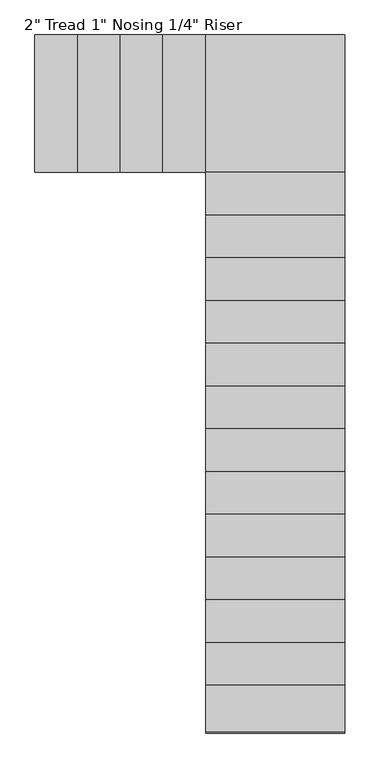
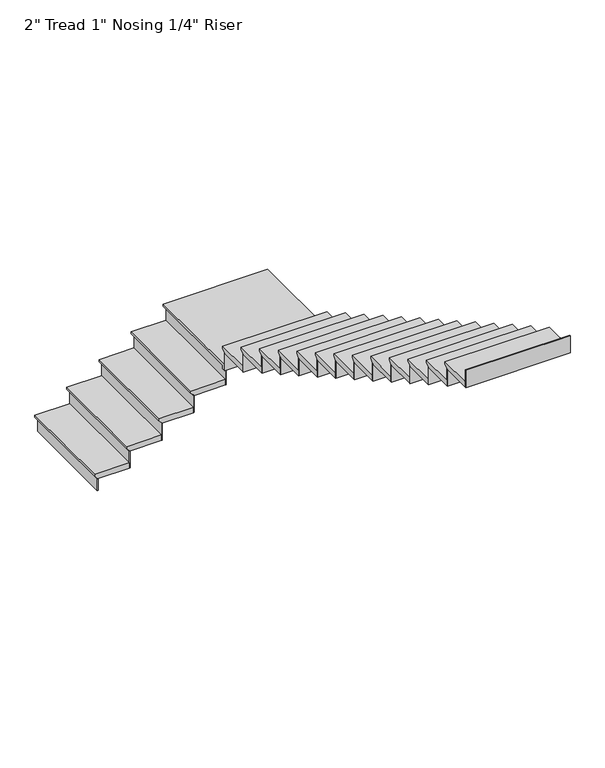
"""IFC4 building model written with IfcOpenShell, lengths in millimetres: stair flight geometry."""

from ifc_helpers import new_model, si_unit, origin, place, context, project, spatial, faceted_brep, source, transform, mapped, element, save


def stair_flight_92322d8c(model_context):
    return source(origin(), model_context, "Body", "Brep", [
        faceted_brep([(-7996.544927, 3130.1909199, 446.1710526), (-7996.544927, 3130.1909199, 465.2210526), (-7996.544927, 4044.5909199, 465.2210526), (-7996.544927, 4044.5909199, 446.1710526), (-7971.144927, 3130.1909199, 420.7710526), (-7971.144927, 4044.5909199, 420.7710526), (-7687.1536588, 3130.1909199, 465.2210526), (-7687.1536588, 4044.5909199, 465.2210526), (-7971.144927, 4044.5909199, 414.4210526), (-7687.1536588, 4044.5909199, 414.4210526), (-7687.1536588, 3130.1909199, 414.4210526), (-7971.144927, 3130.1909199, 414.4210526)], [[[0, 1, 2, 3]], [[4, 0, 3, 5]], [[2, 1, 6, 7]], [[8, 9, 10, 11]], [[2, 7, 9, 8, 5, 3]], [[8, 11, 4, 5]], [[6, 1, 0, 4, 11, 10]], [[7, 6, 10, 9]]]),
        faceted_brep([(-7971.144927, 3130.1909199, 414.4210526), (-7971.144927, 3130.1909199, 304.8), (-7964.794927, 3130.1909199, 304.8), (-7964.794927, 3130.1909199, 414.4210526), (-7971.144927, 4044.5909199, 414.4210526), (-7964.794927, 4044.5909199, 414.4210526), (-7964.794927, 4044.5909199, 304.8), (-7971.144927, 4044.5909199, 304.8)], [[[0, 1, 2, 3]], [[4, 5, 6, 7]], [[1, 0, 4, 7]], [[2, 1, 7, 6]], [[3, 2, 6, 5]], [[0, 3, 5, 4]]]),
        faceted_brep([(-7687.1536588, 3130.1909199, 574.8421053), (-7687.1536588, 3130.1909199, 414.4210526), (-7680.8036588, 3130.1909199, 414.4210526), (-7680.8036588, 3130.1909199, 574.8421053), (-7687.1536588, 4044.5909199, 574.8421053), (-7680.8036588, 4044.5909199, 574.8421053), (-7680.8036588, 4044.5909199, 414.4210526), (-7687.1536588, 4044.5909199, 414.4210526)], [[[0, 1, 2, 3]], [[4, 5, 6, 7]], [[1, 0, 4, 7]], [[2, 1, 7, 6]], [[3, 2, 6, 5]], [[0, 3, 5, 4]]]),
        faceted_brep([(-7712.5536588, 4044.5909199, 625.6421053), (-7712.5536588, 3130.1909199, 625.6421053), (-7403.1623907, 3130.1909199, 625.6421053), (-7403.1623907, 4044.5909199, 625.6421053), (-7687.1536588, 4044.5909199, 574.8421053), (-7403.1623907, 4044.5909199, 574.8421053), (-7403.1623907, 3130.1909199, 574.8421053), (-7687.1536588, 3130.1909199, 574.8421053), (-7687.1536588, 4044.5909199, 581.1921053), (-7712.5536588, 4044.5909199, 606.5921053), (-7687.1536588, 3130.1909199, 581.1921053), (-7712.5536588, 3130.1909199, 606.5921053)], [[[0, 1, 2, 3]], [[4, 5, 6, 7]], [[0, 3, 5, 4, 8, 9]], [[4, 7, 10, 8]], [[2, 1, 11, 10, 7, 6]], [[3, 2, 6, 5]], [[11, 1, 0, 9]], [[10, 11, 9, 8]]]),
        faceted_brep([(-7403.1623907, 3130.1909199, 735.2631579), (-7403.1623907, 3130.1909199, 574.8421053), (-7396.8123907, 3130.1909199, 574.8421053), (-7396.8123907, 3130.1909199, 735.2631579), (-7403.1623907, 4044.5909199, 735.2631579), (-7396.8123907, 4044.5909199, 735.2631579), (-7396.8123907, 4044.5909199, 574.8421053), (-7403.1623907, 4044.5909199, 574.8421053)], [[[0, 1, 2, 3]], [[4, 5, 6, 7]], [[1, 0, 4, 7]], [[2, 1, 7, 6]], [[3, 2, 6, 5]], [[0, 3, 5, 4]]]),
        faceted_brep([(-7428.5623907, 4044.5909199, 786.0631579), (-7428.5623907, 3130.1909199, 786.0631579), (-7119.1711225, 3130.1909199, 786.0631579), (-7119.1711225, 4044.5909199, 786.0631579), (-7403.1623907, 4044.5909199, 735.2631579), (-7119.1711225, 4044.5909199, 735.2631579), (-7119.1711225, 3130.1909199, 735.2631579), (-7403.1623907, 3130.1909199, 735.2631579), (-7403.1623907, 4044.5909199, 741.6131579), (-7428.5623907, 4044.5909199, 767.0131579), (-7403.1623907, 3130.1909199, 741.6131579), (-7428.5623907, 3130.1909199, 767.0131579)], [[[0, 1, 2, 3]], [[4, 5, 6, 7]], [[0, 3, 5, 4, 8, 9]], [[4, 7, 10, 8]], [[2, 1, 11, 10, 7, 6]], [[3, 2, 6, 5]], [[11, 1, 0, 9]], [[10, 11, 9, 8]]]),
        faceted_brep([(-7119.1711225, 3130.1909199, 895.6842105), (-7119.1711225, 3130.1909199, 735.2631579), (-7112.8211225, 3130.1909199, 735.2631579), (-7112.8211225, 3130.1909199, 895.6842105), (-7119.1711225, 4044.5909199, 895.6842105), (-7112.8211225, 4044.5909199, 895.6842105), (-7112.8211225, 4044.5909199, 735.2631579), (-7119.1711225, 4044.5909199, 735.2631579)], [[[0, 1, 2, 3]], [[4, 5, 6, 7]], [[1, 0, 4, 7]], [[2, 1, 7, 6]], [[3, 2, 6, 5]], [[0, 3, 5, 4]]]),
        faceted_brep([(-7144.5711225, 4044.5909199, 946.4842105), (-7144.5711225, 3130.1909199, 946.4842105), (-6835.0860997, 3130.1909199, 946.4842105), (-6835.0860997, 4044.5909199, 946.4842105), (-7119.1711225, 4044.5909199, 895.6842105), (-6835.0860997, 4044.5909199, 895.6842105), (-6835.0860997, 3130.1909199, 895.6842105), (-7119.1711225, 3130.1909199, 895.6842105), (-7119.1711225, 4044.5909199, 902.0342105), (-7144.5711225, 4044.5909199, 927.4342105), (-7119.1711225, 3130.1909199, 902.0342105), (-7144.5711225, 3130.1909199, 927.4342105)], [[[0, 1, 2, 3]], [[4, 5, 6, 7]], [[0, 3, 5, 4, 8, 9]], [[4, 7, 10, 8]], [[2, 1, 11, 10, 7, 6]], [[3, 2, 6, 5]], [[11, 1, 0, 9]], [[10, 11, 9, 8]]]),
        faceted_brep([(-6835.0860997, 3130.1909199, 1056.1052632), (-6835.0860997, 3130.1909199, 895.6842105), (-6828.7360997, 3130.1909199, 895.6842105), (-6828.7360997, 3130.1909199, 1056.1052632), (-6835.0860997, 4044.5909199, 1056.1052632), (-6828.7360997, 4044.5909199, 1056.1052632), (-6828.7360997, 4044.5909199, 895.6842105), (-6835.0860997, 4044.5909199, 895.6842105)], [[[0, 1, 2, 3]], [[4, 5, 6, 7]], [[1, 0, 4, 7]], [[2, 1, 7, 6]], [[3, 2, 6, 5]], [[0, 3, 5, 4]]]),
        faceted_brep([(-5935.2714974, 3104.7909199, 1106.9052632), (-5935.2714974, 4044.5909199, 1106.9052632), (-6860.4860997, 4044.5909199, 1106.9052632), (-6860.4860997, 3104.7909199, 1106.9052632), (-5935.2714974, 4044.5909199, 1056.1052632), (-5935.2714974, 3104.7909199, 1056.1052632), (-6860.4860997, 3104.7909199, 1056.1052632), (-6860.4860997, 3130.1909199, 1056.1052632), (-6835.0860997, 3130.1909199, 1056.1052632), (-6835.0860997, 4044.5909199, 1056.1052632), (-6835.0860997, 4044.5909199, 1062.4552632), (-6860.4860997, 4044.5909199, 1087.8552632), (-6835.0860997, 3130.1909199, 1062.4552632), (-6860.4860997, 3130.1909199, 1087.8552632)], [[[0, 1, 2, 3]], [[4, 5, 6, 7, 8, 9]], [[1, 0, 5, 4]], [[2, 1, 4, 9, 10, 11]], [[9, 8, 12, 10]], [[8, 7, 13, 12]], [[3, 2, 11, 13, 7, 6]], [[0, 3, 6, 5]], [[11, 10, 12, 13]]]),
        faceted_brep([(-6860.4860997, 3104.7909199, 1216.5263158), (-6860.4860997, 3104.7909199, 1056.1052632), (-6860.4860997, 3098.4409199, 1056.1052632), (-6860.4860997, 3098.4409199, 1216.5263158), (-5935.2714974, 3104.7909199, 1216.5263158), (-5935.2714974, 3098.4409199, 1216.5263158), (-5935.2714974, 3098.4409199, 1056.1052632), (-5935.2714974, 3104.7909199, 1056.1052632)], [[[0, 1, 2, 3]], [[4, 5, 6, 7]], [[1, 0, 4, 7]], [[2, 1, 7, 6]], [[3, 2, 6, 5]], [[0, 3, 5, 4]]]),
        faceted_brep([(-5935.2714974, 3130.1909199, 1267.3263158), (-6860.4860997, 3130.1909199, 1267.3263158), (-6860.4860997, 2820.3109199, 1267.3263158), (-5935.2714974, 2820.3109199, 1267.3263158), (-5935.2714974, 3104.7909199, 1216.5263158), (-5935.2714974, 2820.3109199, 1216.5263158), (-6860.4860997, 2820.3109199, 1216.5263158), (-6860.4860997, 3104.7909199, 1216.5263158), (-5935.2714974, 3104.7909199, 1222.8763158), (-5935.2714974, 3130.1909199, 1248.2763158), (-6860.4860997, 3104.7909199, 1222.8763158), (-6860.4860997, 3130.1909199, 1248.2763158)], [[[0, 1, 2, 3]], [[4, 5, 6, 7]], [[0, 3, 5, 4, 8, 9]], [[4, 7, 10, 8]], [[2, 1, 11, 10, 7, 6]], [[3, 2, 6, 5]], [[11, 1, 0, 9]], [[10, 11, 9, 8]]]),
        faceted_brep([(-6860.4860997, 2820.3109199, 1376.9473684), (-6860.4860997, 2820.3109199, 1216.5263158), (-6860.4860997, 2813.9609199, 1216.5263158), (-6860.4860997, 2813.9609199, 1376.9473684), (-5935.2714974, 2820.3109199, 1376.9473684), (-5935.2714974, 2813.9609199, 1376.9473684), (-5935.2714974, 2813.9609199, 1216.5263158), (-5935.2714974, 2820.3109199, 1216.5263158)], [[[0, 1, 2, 3]], [[4, 5, 6, 7]], [[1, 0, 4, 7]], [[2, 1, 7, 6]], [[3, 2, 6, 5]], [[0, 3, 5, 4]]]),
        faceted_brep([(-5935.2714974, 2845.7109199, 1427.7473684), (-6860.4860997, 2845.7109199, 1427.7473684), (-6860.4860997, 2535.8309199, 1427.7473684), (-5935.2714974, 2535.8309199, 1427.7473684), (-5935.2714974, 2820.3109199, 1376.9473684), (-5935.2714974, 2535.8309199, 1376.9473684), (-6860.4860997, 2535.8309199, 1376.9473684), (-6860.4860997, 2820.3109199, 1376.9473684), (-5935.2714974, 2820.3109199, 1383.2973684), (-5935.2714974, 2845.7109199, 1408.6973684), (-6860.4860997, 2820.3109199, 1383.2973684), (-6860.4860997, 2845.7109199, 1408.6973684)], [[[0, 1, 2, 3]], [[4, 5, 6, 7]], [[0, 3, 5, 4, 8, 9]], [[4, 7, 10, 8]], [[2, 1, 11, 10, 7, 6]], [[3, 2, 6, 5]], [[11, 1, 0, 9]], [[10, 11, 9, 8]]]),
        faceted_brep([(-6860.4860997, 2535.8309199, 1537.3684211), (-6860.4860997, 2535.8309199, 1376.9473684), (-6860.4860997, 2529.4809199, 1376.9473684), (-6860.4860997, 2529.4809199, 1537.3684211), (-5935.2714974, 2535.8309199, 1537.3684211), (-5935.2714974, 2529.4809199, 1537.3684211), (-5935.2714974, 2529.4809199, 1376.9473684), (-5935.2714974, 2535.8309199, 1376.9473684)], [[[0, 1, 2, 3]], [[4, 5, 6, 7]], [[1, 0, 4, 7]], [[2, 1, 7, 6]], [[3, 2, 6, 5]], [[0, 3, 5, 4]]]),
        faceted_brep([(-5935.2714974, 2561.2309199, 1588.1684211), (-6860.4860997, 2561.2309199, 1588.1684211), (-6860.4860997, 2251.3509199, 1588.1684211), (-5935.2714974, 2251.3509199, 1588.1684211), (-5935.2714974, 2535.8309199, 1537.3684211), (-5935.2714974, 2251.3509199, 1537.3684211), (-6860.4860997, 2251.3509199, 1537.3684211), (-6860.4860997, 2535.8309199, 1537.3684211), (-5935.2714974, 2535.8309199, 1543.7184211), (-5935.2714974, 2561.2309199, 1569.1184211), (-6860.4860997, 2535.8309199, 1543.7184211), (-6860.4860997, 2561.2309199, 1569.1184211)], [[[0, 1, 2, 3]], [[4, 5, 6, 7]], [[0, 3, 5, 4, 8, 9]], [[4, 7, 10, 8]], [[2, 1, 11, 10, 7, 6]], [[3, 2, 6, 5]], [[11, 1, 0, 9]], [[10, 11, 9, 8]]]),
        faceted_brep([(-6860.4860997, 2251.3509199, 1697.7894737), (-6860.4860997, 2251.3509199, 1537.3684211), (-6860.4860997, 2245.0009199, 1537.3684211), (-6860.4860997, 2245.0009199, 1697.7894737), (-5935.2714974, 2251.3509199, 1697.7894737), (-5935.2714974, 2245.0009199, 1697.7894737), (-5935.2714974, 2245.0009199, 1537.3684211), (-5935.2714974, 2251.3509199, 1537.3684211)], [[[0, 1, 2, 3]], [[4, 5, 6, 7]], [[1, 0, 4, 7]], [[2, 1, 7, 6]], [[3, 2, 6, 5]], [[0, 3, 5, 4]]]),
        faceted_brep([(-5935.2714974, 2276.7509199, 1748.5894737), (-6860.4860997, 2276.7509199, 1748.5894737), (-6860.4860997, 1966.8709199, 1748.5894737), (-5935.2714974, 1966.8709199, 1748.5894737), (-5935.2714974, 2251.3509199, 1697.7894737), (-5935.2714974, 1966.8709199, 1697.7894737), (-6860.4860997, 1966.8709199, 1697.7894737), (-6860.4860997, 2251.3509199, 1697.7894737), (-5935.2714974, 2251.3509199, 1704.1394737), (-5935.2714974, 2276.7509199, 1729.5394737), (-6860.4860997, 2251.3509199, 1704.1394737), (-6860.4860997, 2276.7509199, 1729.5394737)], [[[0, 1, 2, 3]], [[4, 5, 6, 7]], [[0, 3, 5, 4, 8, 9]], [[4, 7, 10, 8]], [[2, 1, 11, 10, 7, 6]], [[3, 2, 6, 5]], [[11, 1, 0, 9]], [[10, 11, 9, 8]]]),
        faceted_brep([(-6860.4860997, 1966.8709199, 1858.2105263), (-6860.4860997, 1966.8709199, 1697.7894737), (-6860.4860997, 1960.5209199, 1697.7894737), (-6860.4860997, 1960.5209199, 1858.2105263), (-5935.2714974, 1966.8709199, 1858.2105263), (-5935.2714974, 1960.5209199, 1858.2105263), (-5935.2714974, 1960.5209199, 1697.7894737), (-5935.2714974, 1966.8709199, 1697.7894737)], [[[0, 1, 2, 3]], [[4, 5, 6, 7]], [[1, 0, 4, 7]], [[2, 1, 7, 6]], [[3, 2, 6, 5]], [[0, 3, 5, 4]]]),
        faceted_brep([(-5935.2714974, 1992.2709199, 1909.0105263), (-6860.4860997, 1992.2709199, 1909.0105263), (-6860.4860997, 1682.3909199, 1909.0105263), (-5935.2714974, 1682.3909199, 1909.0105263), (-5935.2714974, 1966.8709199, 1858.2105263), (-5935.2714974, 1682.3909199, 1858.2105263), (-6860.4860997, 1682.3909199, 1858.2105263), (-6860.4860997, 1966.8709199, 1858.2105263), (-5935.2714974, 1966.8709199, 1864.5605263), (-5935.2714974, 1992.2709199, 1889.9605263), (-6860.4860997, 1966.8709199, 1864.5605263), (-6860.4860997, 1992.2709199, 1889.9605263)], [[[0, 1, 2, 3]], [[4, 5, 6, 7]], [[0, 3, 5, 4, 8, 9]], [[4, 7, 10, 8]], [[2, 1, 11, 10, 7, 6]], [[3, 2, 6, 5]], [[11, 1, 0, 9]], [[10, 11, 9, 8]]]),
        faceted_brep([(-6860.4860997, 1682.3909199, 2018.6315789), (-6860.4860997, 1682.3909199, 1858.2105263), (-6860.4860997, 1676.0409199, 1858.2105263), (-6860.4860997, 1676.0409199, 2018.6315789), (-5935.2714974, 1682.3909199, 2018.6315789), (-5935.2714974, 1676.0409199, 2018.6315789), (-5935.2714974, 1676.0409199, 1858.2105263), (-5935.2714974, 1682.3909199, 1858.2105263)], [[[0, 1, 2, 3]], [[4, 5, 6, 7]], [[1, 0, 4, 7]], [[2, 1, 7, 6]], [[3, 2, 6, 5]], [[0, 3, 5, 4]]]),
        faceted_brep([(-5935.2714974, 1707.7909199, 2069.4315789), (-6860.4860997, 1707.7909199, 2069.4315789), (-6860.4860997, 1397.9109198, 2069.4315789), (-5935.2714974, 1397.9109198, 2069.4315789), (-5935.2714974, 1682.3909199, 2018.6315789), (-5935.2714974, 1397.9109198, 2018.6315789), (-6860.4860997, 1397.9109198, 2018.6315789), (-6860.4860997, 1682.3909199, 2018.6315789), (-5935.2714974, 1682.3909199, 2024.9815789), (-5935.2714974, 1707.7909199, 2050.3815789), (-6860.4860997, 1682.3909199, 2024.9815789), (-6860.4860997, 1707.7909199, 2050.3815789)], [[[0, 1, 2, 3]], [[4, 5, 6, 7]], [[0, 3, 5, 4, 8, 9]], [[4, 7, 10, 8]], [[2, 1, 11, 10, 7, 6]], [[3, 2, 6, 5]], [[11, 1, 0, 9]], [[10, 11, 9, 8]]]),
        faceted_brep([(-6860.4860997, 1397.9109199, 2179.0526316), (-6860.4860997, 1397.9109199, 2018.6315789), (-6860.4860997, 1391.5609199, 2018.6315789), (-6860.4860997, 1391.5609199, 2179.0526316), (-5935.2714974, 1397.9109199, 2179.0526316), (-5935.2714974, 1391.5609199, 2179.0526316), (-5935.2714974, 1391.5609199, 2018.6315789), (-5935.2714974, 1397.9109199, 2018.6315789)], [[[0, 1, 2, 3]], [[4, 5, 6, 7]], [[1, 0, 4, 7]], [[2, 1, 7, 6]], [[3, 2, 6, 5]], [[0, 3, 5, 4]]]),
        faceted_brep([(-5935.2714974, 1423.3109199, 2229.8526316), (-6860.4860997, 1423.3109199, 2229.8526316), (-6860.4860997, 1113.4309198, 2229.8526316), (-5935.2714974, 1113.4309198, 2229.8526316), (-5935.2714974, 1397.9109199, 2179.0526316), (-5935.2714974, 1113.4309198, 2179.0526316), (-6860.4860997, 1113.4309198, 2179.0526316), (-6860.4860997, 1397.9109199, 2179.0526316), (-5935.2714974, 1397.9109199, 2185.4026316), (-5935.2714974, 1423.3109199, 2210.8026316), (-6860.4860997, 1397.9109199, 2185.4026316), (-6860.4860997, 1423.3109199, 2210.8026316)], [[[0, 1, 2, 3]], [[4, 5, 6, 7]], [[0, 3, 5, 4, 8, 9]], [[4, 7, 10, 8]], [[2, 1, 11, 10, 7, 6]], [[3, 2, 6, 5]], [[11, 1, 0, 9]], [[10, 11, 9, 8]]]),
        faceted_brep([(-6860.4860997, 1113.4309199, 2339.4736842), (-6860.4860997, 1113.4309199, 2179.0526316), (-6860.4860997, 1107.0809199, 2179.0526316), (-6860.4860997, 1107.0809199, 2339.4736842), (-5935.2714974, 1113.4309199, 2339.4736842), (-5935.2714974, 1107.0809199, 2339.4736842), (-5935.2714974, 1107.0809199, 2179.0526316), (-5935.2714974, 1113.4309199, 2179.0526316)], [[[0, 1, 2, 3]], [[4, 5, 6, 7]], [[1, 0, 4, 7]], [[2, 1, 7, 6]], [[3, 2, 6, 5]], [[0, 3, 5, 4]]]),
        faceted_brep([(-5935.2714974, 1138.8309199, 2390.2736842), (-6860.4860997, 1138.8309199, 2390.2736842), (-6860.4860997, 828.9509198, 2390.2736842), (-5935.2714974, 828.9509198, 2390.2736842), (-5935.2714974, 1113.4309199, 2339.4736842), (-5935.2714974, 828.9509198, 2339.4736842), (-6860.4860997, 828.9509198, 2339.4736842), (-6860.4860997, 1113.4309199, 2339.4736842), (-5935.2714974, 1113.4309199, 2345.8236842), (-5935.2714974, 1138.8309199, 2371.2236842), (-6860.4860997, 1113.4309199, 2345.8236842), (-6860.4860997, 1138.8309199, 2371.2236842)], [[[0, 1, 2, 3]], [[4, 5, 6, 7]], [[0, 3, 5, 4, 8, 9]], [[4, 7, 10, 8]], [[2, 1, 11, 10, 7, 6]], [[3, 2, 6, 5]], [[11, 1, 0, 9]], [[10, 11, 9, 8]]]),
        faceted_brep([(-6860.4860997, 828.9509199, 2499.8947368), (-6860.4860997, 828.9509199, 2339.4736842), (-6860.4860997, 822.6009199, 2339.4736842), (-6860.4860997, 822.6009199, 2499.8947368), (-5935.2714974, 828.9509199, 2499.8947368), (-5935.2714974, 822.6009199, 2499.8947368), (-5935.2714974, 822.6009199, 2339.4736842), (-5935.2714974, 828.9509199, 2339.4736842)], [[[0, 1, 2, 3]], [[4, 5, 6, 7]], [[1, 0, 4, 7]], [[2, 1, 7, 6]], [[3, 2, 6, 5]], [[0, 3, 5, 4]]]),
        faceted_brep([(-5935.2714974, 854.3509199, 2550.6947368), (-6860.4860997, 854.3509199, 2550.6947368), (-6860.4860997, 544.4709198, 2550.6947368), (-5935.2714974, 544.4709198, 2550.6947368), (-5935.2714974, 828.9509199, 2499.8947368), (-5935.2714974, 544.4709198, 2499.8947368), (-6860.4860997, 544.4709198, 2499.8947368), (-6860.4860997, 828.9509199, 2499.8947368), (-5935.2714974, 828.9509199, 2506.2447368), (-5935.2714974, 854.3509199, 2531.6447368), (-6860.4860997, 828.9509199, 2506.2447368), (-6860.4860997, 854.3509199, 2531.6447368)], [[[0, 1, 2, 3]], [[4, 5, 6, 7]], [[0, 3, 5, 4, 8, 9]], [[4, 7, 10, 8]], [[2, 1, 11, 10, 7, 6]], [[3, 2, 6, 5]], [[11, 1, 0, 9]], [[10, 11, 9, 8]]]),
        faceted_brep([(-6860.4860997, 544.4709198, 2660.3157895), (-6860.4860997, 544.4709198, 2499.8947368), (-6860.4860997, 538.1209198, 2499.8947368), (-6860.4860997, 538.1209198, 2660.3157895), (-5935.2714974, 544.4709198, 2660.3157895), (-5935.2714974, 538.1209198, 2660.3157895), (-5935.2714974, 538.1209198, 2499.8947368), (-5935.2714974, 544.4709198, 2499.8947368)], [[[0, 1, 2, 3]], [[4, 5, 6, 7]], [[1, 0, 4, 7]], [[2, 1, 7, 6]], [[3, 2, 6, 5]], [[0, 3, 5, 4]]]),
        faceted_brep([(-5935.2714974, 569.8709198, 2711.1157895), (-6860.4860997, 569.8709198, 2711.1157895), (-6860.4860997, 260.0107636, 2711.1157895), (-5935.2714974, 260.0107636, 2711.1157895), (-5935.2714974, 544.4709198, 2660.3157895), (-5935.2714974, 260.0107636, 2660.3157895), (-6860.4860997, 260.0107636, 2660.3157895), (-6860.4860997, 544.4709198, 2660.3157895), (-5935.2714974, 544.4709198, 2666.6657895), (-5935.2714974, 569.8709198, 2692.0657895), (-6860.4860997, 544.4709198, 2666.6657895), (-6860.4860997, 569.8709198, 2692.0657895)], [[[0, 1, 2, 3]], [[4, 5, 6, 7]], [[0, 3, 5, 4, 8, 9]], [[4, 7, 10, 8]], [[2, 1, 11, 10, 7, 6]], [[3, 2, 6, 5]], [[11, 1, 0, 9]], [[10, 11, 9, 8]]]),
        faceted_brep([(-6860.4860997, 260.0107636, 2820.7368421), (-6860.4860997, 260.0107636, 2660.3157895), (-6860.4860997, 253.6607636, 2660.3157895), (-6860.4860997, 253.6607636, 2820.7368421), (-5935.2714974, 260.0107636, 2820.7368421), (-5935.2714974, 253.6607636, 2820.7368421), (-5935.2714974, 253.6607636, 2660.3157895), (-5935.2714974, 260.0107636, 2660.3157895)], [[[0, 1, 2, 3]], [[4, 5, 6, 7]], [[1, 0, 4, 7]], [[2, 1, 7, 6]], [[3, 2, 6, 5]], [[0, 3, 5, 4]]]),
        faceted_brep([(-5935.2714974, 285.4107636, 2871.5368421), (-6860.4860997, 285.4107636, 2871.5368421), (-6860.4860997, -24.4493927, 2871.5368421), (-5935.2714974, -24.4493927, 2871.5368421), (-5935.2714974, 260.0107636, 2820.7368421), (-5935.2714974, -24.4493927, 2820.7368421), (-6860.4860997, -24.4493927, 2820.7368421), (-6860.4860997, 260.0107636, 2820.7368421), (-5935.2714974, 260.0107636, 2827.0868421), (-5935.2714974, 285.4107636, 2852.4868421), (-6860.4860997, 260.0107636, 2827.0868421), (-6860.4860997, 285.4107636, 2852.4868421)], [[[0, 1, 2, 3]], [[4, 5, 6, 7]], [[0, 3, 5, 4, 8, 9]], [[4, 7, 10, 8]], [[2, 1, 11, 10, 7, 6]], [[3, 2, 6, 5]], [[11, 1, 0, 9]], [[10, 11, 9, 8]]]),
        faceted_brep([(-6860.4860997, -24.4493927, 2981.1578947), (-6860.4860997, -24.4493927, 2820.7368421), (-6860.4860997, -30.7993927, 2820.7368421), (-6860.4860997, -30.7993927, 2981.1578947), (-5935.2714974, -24.4493927, 2981.1578947), (-5935.2714974, -30.7993927, 2981.1578947), (-5935.2714974, -30.7993927, 2820.7368421), (-5935.2714974, -24.4493927, 2820.7368421)], [[[0, 1, 2, 3]], [[4, 5, 6, 7]], [[1, 0, 4, 7]], [[2, 1, 7, 6]], [[3, 2, 6, 5]], [[0, 3, 5, 4]]]),
        faceted_brep([(-5935.2714974, 0.9506073, 3031.9578947), (-6860.4860997, 0.9506073, 3031.9578947), (-6860.4860997, -308.9095489, 3031.9578947), (-5935.2714974, -308.9095489, 3031.9578947), (-5935.2714974, -24.4493927, 2981.1578947), (-5935.2714974, -308.9095489, 2981.1578947), (-6860.4860997, -308.9095489, 2981.1578947), (-6860.4860997, -24.4493927, 2981.1578947), (-5935.2714974, -24.4493927, 2987.5078947), (-5935.2714974, 0.9506073, 3012.9078947), (-6860.4860997, -24.4493927, 2987.5078947), (-6860.4860997, 0.9506073, 3012.9078947)], [[[0, 1, 2, 3]], [[4, 5, 6, 7]], [[0, 3, 5, 4, 8, 9]], [[4, 7, 10, 8]], [[2, 1, 11, 10, 7, 6]], [[3, 2, 6, 5]], [[11, 1, 0, 9]], [[10, 11, 9, 8]]]),
        faceted_brep([(-6860.4860997, -308.9095489, 3141.5789474), (-6860.4860997, -308.9095489, 2981.1578947), (-6860.4860997, -315.2595489, 2981.1578947), (-6860.4860997, -315.2595489, 3141.5789474), (-5935.2714974, -308.9095489, 3141.5789474), (-5935.2714974, -315.2595489, 3141.5789474), (-5935.2714974, -315.2595489, 2981.1578947), (-5935.2714974, -308.9095489, 2981.1578947)], [[[0, 1, 2, 3]], [[4, 5, 6, 7]], [[1, 0, 4, 7]], [[2, 1, 7, 6]], [[3, 2, 6, 5]], [[0, 3, 5, 4]]]),
        faceted_brep([(-6860.4860997, -593.3697052, 3302.0), (-6860.4860997, -593.3697052, 3141.5789474), (-6860.4860997, -599.7197052, 3141.5789474), (-6860.4860997, -599.7197052, 3302.0), (-5935.2714974, -593.3697052, 3302.0), (-5935.2714974, -599.7197052, 3302.0), (-5935.2714974, -599.7197052, 3141.5789474), (-5935.2714974, -593.3697052, 3141.5789474)], [[[0, 1, 2, 3]], [[4, 5, 6, 7]], [[1, 0, 4, 7]], [[2, 1, 7, 6]], [[3, 2, 6, 5]], [[0, 3, 5, 4]]]),
        faceted_brep([(-5935.2714974, -283.5095489, 3192.3789474), (-6860.4860997, -283.5095489, 3192.3789474), (-6860.4860997, -593.3697052, 3192.3789474), (-5935.2714974, -593.3697052, 3192.3789474), (-5935.2714974, -308.9095489, 3141.5789474), (-5935.2714974, -593.3697052, 3141.5789474), (-6860.4860997, -593.3697052, 3141.5789474), (-6860.4860997, -308.9095489, 3141.5789474), (-5935.2714974, -308.9095489, 3147.9289474), (-5935.2714974, -283.5095489, 3173.3289474), (-6860.4860997, -308.9095489, 3147.9289474), (-6860.4860997, -283.5095489, 3173.3289474)], [[[0, 1, 2, 3]], [[4, 5, 6, 7]], [[0, 3, 5, 4, 8, 9]], [[4, 7, 10, 8]], [[2, 1, 11, 10, 7, 6]], [[3, 2, 6, 5]], [[11, 1, 0, 9]], [[10, 11, 9, 8]]]),
    ])


if __name__ == "__main__":
    model = new_model("IFC4")
    model_context = context("Model", 3, world=origin())
    ifc_project = project(units=[si_unit("LENGTHUNIT", "METRE", prefix="MILLI")], contexts=[model_context])
    site = spatial("IfcSite", under=ifc_project)
    building = spatial("IfcBuilding", under=site)
    placement = place(None, origin())
    stair_flight_shape = stair_flight_92322d8c(model_context)
    element("IfcStairFlight", 1, ObjectType="2\" Tread 1\" Nosing 1/4\" Riser", at=placement, inside=building, context=model_context, shape_type="MappedRepresentation", body=[
        mapped(stair_flight_shape, transform((0.0, 0.0, 0.0), x_axis=(1.0, 0.0, 0.0), y_axis=(0.0, 1.0, 0.0), z_axis=(0.0, 0.0, 1.0))),
    ])
    save(model, "model.ifc")
